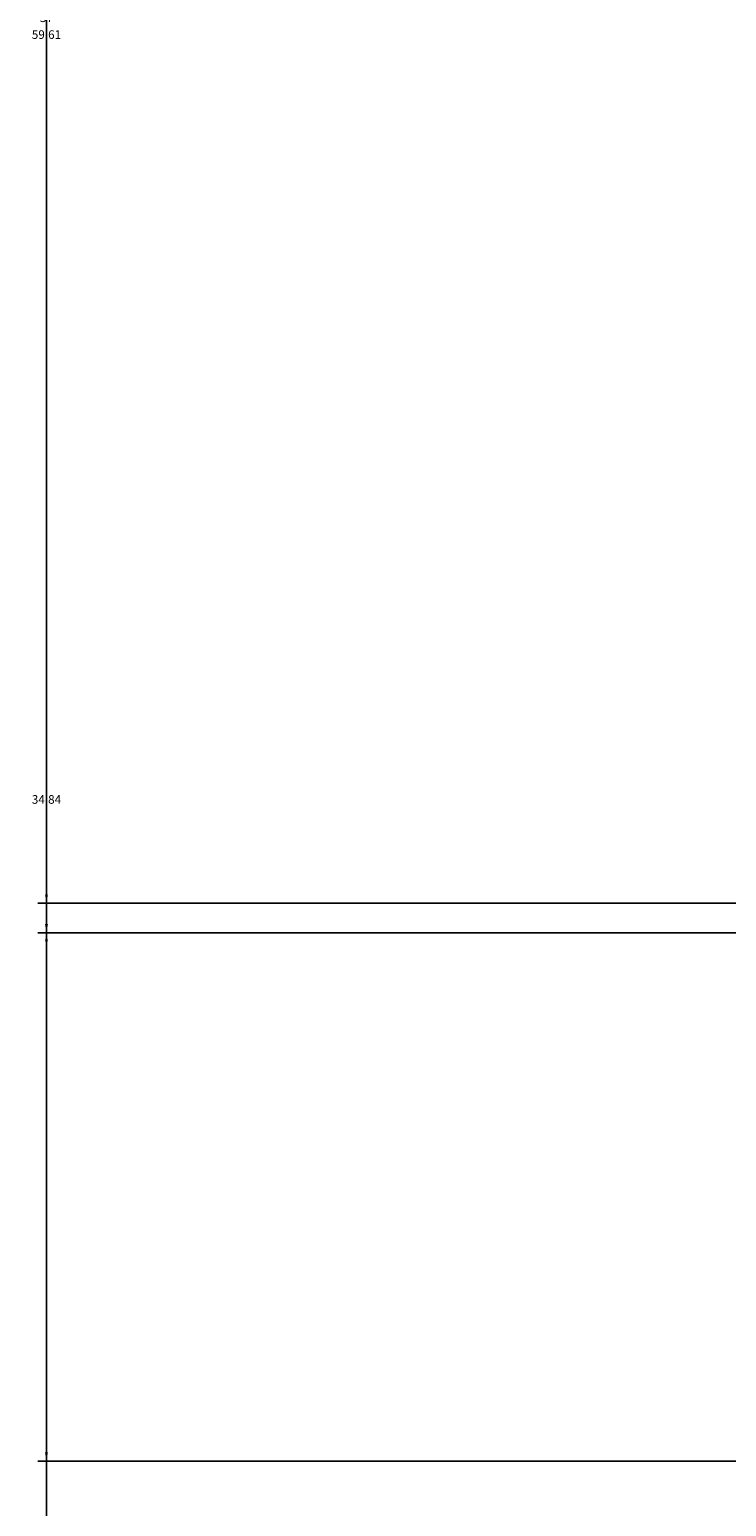
# Model space of a CAD drawing. Units: inches. Extents: x -12 to 334, y -10 to 186.
# Tile 3 of 77: x -12 to 3, y 49 to 79. Entities that reach past the tile are written whole.
import ezdxf

# ---------------------------------------------------------------- set-up
doc = ezdxf.new("R2010")
doc.units = ezdxf.units.IN
doc.header["$MEASUREMENT"] = 0
doc.layers.add('M-DIMS', color=2, linetype='Continuous', lineweight=18)
doc.styles.get("Standard").update_dxf_attribs({"font": 'arial.ttf'})
doc.dimstyles.get("Standard").update_dxf_attribs({"dimtxt": 0.18, "dimasz": 0.18, "dimexe": 0.18, "dimexo": 0.0625, "dimgap": 0.09, "dimtad": 0, "dimtih": 1, "dimtoh": 1, "dimdec": 4, "dimzin": 0, "dimdsep": 46, "dimtxsty": 'Standard', "dimcen": 0.09, "dimadec": 0, "dimazin": 0, "dimtfac": 1, "dimtdec": 4, "dimtofl": 0, "dimtmove": 0, "dimatfit": 3, "dimfxl": 1, "dimtolj": 1, "dimtzin": 0, "dimarcsym": 0})

# ---------------------------------------------------------------- blocks, each defined once
blk = doc.blocks.new('*D6')
at = {"layer": 'Defpoints', "color": 0, "transparency": 16777216}
for p in [(-11.174, 60.487), (23.581, 60.487), (32.1, 33.675)]:
    blk.add_point(p, dxfattribs=at)
at = {"layer": 'M-DIMS', "color": 0, "lineweight": -2, "transparency": 16777216}
for p, q in [((23.518, 60.487), (-11.354, 60.487)), ((-11.174, 60.307), (-11.174, 47.263)), ((-11.174, 33.855), (-11.174, 46.899)), ((32.038, 33.675), (-11.354, 33.675))]:
    blk.add_line(p, q, dxfattribs=at)
at = {"layer": 'M-DIMS', "color": 0, "transparency": 16777216}
for points in [[(-11.204, 60.307), (-11.144, 60.307), (-11.174, 60.487)], [(-11.204, 33.855), (-11.144, 33.855), (-11.174, 33.675)]]:
    blk.add_solid(points, dxfattribs=at)
at = {"layer": 'M-DIMS', "color": 0, "transparency": 16777216, "insert": (-11.174, 47.081), "char_height": 0.18, "attachment_point": 5}
blk.add_mtext('\\A1;26.81', dxfattribs=at)
blk = doc.blocks.new('*D7')
at = {"layer": 'Defpoints', "color": 0, "transparency": 16777216}
for p in [(-11.174, 100.896), (23.581, 100.896), (23.581, 60.487)]:
    blk.add_point(p, dxfattribs=at)
at = {"layer": 'M-DIMS', "color": 0, "lineweight": -2, "transparency": 16777216}
for p, q in [((23.518, 100.896), (-11.354, 100.896)), ((-11.174, 100.716), (-11.174, 80.873)), ((-11.174, 60.667), (-11.174, 80.51)), ((23.518, 60.487), (-11.354, 60.487))]:
    blk.add_line(p, q, dxfattribs=at)
at = {"layer": 'M-DIMS', "color": 0, "transparency": 16777216}
for points in [[(-11.204, 100.716), (-11.144, 100.716), (-11.174, 100.896)], [(-11.204, 60.667), (-11.144, 60.667), (-11.174, 60.487)]]:
    blk.add_solid(points, dxfattribs=at)
at = {"layer": 'M-DIMS', "color": 0, "transparency": 16777216, "insert": (-11.174, 80.692), "char_height": 0.18, "attachment_point": 5}
blk.add_mtext('\\A1;40.41', dxfattribs=at)
blk = doc.blocks.new('*D14')
at = {"layer": 'Defpoints', "color": 0, "transparency": 16777216}
for p in [(63.5, 109.058), (-11.174, 49.45), (64.207, 49.45)]:
    blk.add_point(p, dxfattribs=at)
at = {"layer": 'M-DIMS', "color": 0, "lineweight": -2, "transparency": 16777216}
for p, q in [((63.438, 109.058), (-11.354, 109.058)), ((-11.174, 108.878), (-11.174, 79.436)), ((-11.174, 49.63), (-11.174, 79.072)), ((64.144, 49.45), (-11.354, 49.45))]:
    blk.add_line(p, q, dxfattribs=at)
at = {"layer": 'M-DIMS', "color": 0, "transparency": 16777216}
for points in [[(-11.204, 108.878), (-11.144, 108.878), (-11.174, 109.058)], [(-11.204, 49.63), (-11.144, 49.63), (-11.174, 49.45)]]:
    blk.add_solid(points, dxfattribs=at)
at = {"layer": 'M-DIMS', "color": 0, "transparency": 16777216, "insert": (-11.174, 79.254), "char_height": 0.18, "attachment_point": 5}
blk.add_mtext('\\A1;59.61', dxfattribs=at)
blk = doc.blocks.new('*D35')
at = {"layer": 'Defpoints', "color": 0, "transparency": 16777216}
for p in [(216.428, 98.108), (-11.174, 61.105), (216.428, 61.105)]:
    blk.add_point(p, dxfattribs=at)
at = {"layer": 'M-DIMS', "color": 0, "lineweight": -2, "transparency": 16777216}
for p, q in [((216.365, 98.108), (-11.354, 98.108)), ((-11.174, 97.928), (-11.174, 79.788)), ((-11.174, 61.285), (-11.174, 79.424)), ((216.365, 61.105), (-11.354, 61.105))]:
    blk.add_line(p, q, dxfattribs=at)
at = {"layer": 'M-DIMS', "color": 0, "transparency": 16777216}
for points in [[(-11.204, 97.928), (-11.144, 97.928), (-11.174, 98.108)], [(-11.204, 61.285), (-11.144, 61.285), (-11.174, 61.105)]]:
    blk.add_solid(points, dxfattribs=at)
at = {"layer": 'M-DIMS', "color": 0, "transparency": 16777216, "insert": (-11.174, 79.606), "char_height": 0.18, "attachment_point": 5}
blk.add_mtext('\\A1;37', dxfattribs=at)
blk = doc.blocks.new('*D39')
at = {"layer": 'Defpoints', "color": 0, "transparency": 16777216}
for p in [(279.726, 80.692), (-11.174, 45.854), (269.381, 45.854)]:
    blk.add_point(p, dxfattribs=at)
at = {"layer": 'M-DIMS', "color": 0, "lineweight": -2, "transparency": 16777216}
for p, q in [((279.664, 80.692), (-11.354, 80.692)), ((-11.174, 80.512), (-11.174, 63.455)), ((-11.174, 46.034), (-11.174, 63.091)), ((269.318, 45.854), (-11.354, 45.854))]:
    blk.add_line(p, q, dxfattribs=at)
at = {"layer": 'M-DIMS', "color": 0, "transparency": 16777216}
for points in [[(-11.204, 80.512), (-11.144, 80.512), (-11.174, 80.692)], [(-11.204, 46.034), (-11.144, 46.034), (-11.174, 45.854)]]:
    blk.add_solid(points, dxfattribs=at)
at = {"layer": 'M-DIMS', "color": 0, "transparency": 16777216, "insert": (-11.174, 63.273), "char_height": 0.18, "attachment_point": 5}
blk.add_mtext('\\A1;34.84', dxfattribs=at)

msp = doc.modelspace()

# ---------------------------------------------------------------- dimensions: what is measured, and where the dimension line sits
at = {"layer": 'M-DIMS'}
for base, p1, p2, override, picture, middle in [((-11.1736, 49.4497), (63.5, 109.0583), (64.2068, 49.4497), {"dimdec": 2, "dimlfac": 1, "dimrnd": 0, "dimzin": 0, "dimdsep": 46, "dimlunit": 2}, '*D14', (-11.1735, 79.254)), ((-11.1736, 100.8958), (23.5807, 60.4872), (23.5807, 100.8958), {"dimdec": 2, "dimlfac": 1, "dimrnd": 0, "dimzin": 0, "dimdsep": 46, "dimlunit": 2}, '*D7', (-11.1735, 80.6915)), ((-11.1736, 61.1045), (216.4278, 98.1081), (216.4278, 61.1045), {"dimdec": 0, "dimlfac": 1, "dimrnd": 0, "dimzin": 0, "dimdsep": 46, "dimlunit": 2}, '*D35', (-11.1735, 79.6063)), ((-11.1736, 45.8541), (279.7263, 80.6915), (269.3808, 45.8541), {"dimdec": 2, "dimlfac": 1, "dimrnd": 0, "dimzin": 0, "dimdsep": 46, "dimlunit": 2}, '*D39', (-11.1735, 63.2728)), ((-11.1736, 60.4872), (32.1002, 33.6752), (23.5807, 60.4872), {"dimdec": 2, "dimlfac": 1, "dimrnd": 0, "dimzin": 0, "dimdsep": 46, "dimlunit": 2}, '*D6', (-11.1735, 47.0812))]:
    dim = msp.add_linear_dim(base=base, p1=p1, p2=p2, angle=90, dimstyle='Standard', override=override, dxfattribs=at)
    dim.commit()
    dim.dimension.update_dxf_attribs({"geometry": picture, "text_midpoint": middle})

doc.saveas('drawing.dxf')
